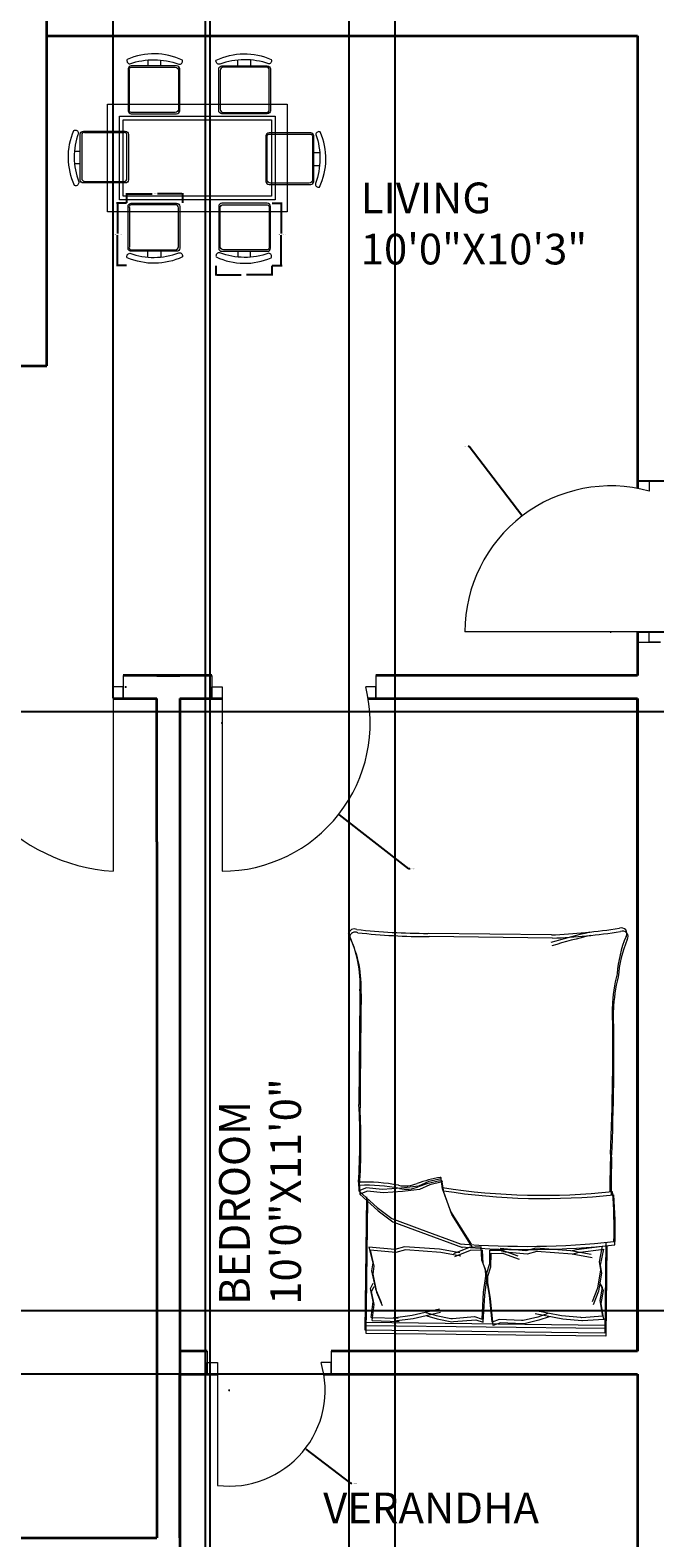
# Model space of a CAD drawing. Units: inches. Extents: x 1721 to 2510, y 1544 to 2360.
# Tile 3 of 10: x 1924 to 2046, y 1693 to 1988. Entities that reach past the tile are written whole.
import ezdxf

# ---------------------------------------------------------------- set-up
doc = ezdxf.new("R2010")
doc.units = ezdxf.units.IN
for name, color, linetype, lineweight in [('A-ANNO-DIMS', 2, 'Continuous', 18), ('A-AREA-IDEN', 7, 'Continuous', 18), ('A-DOOR', 3, 'Continuous', 18), ('A-FURN', 8, 'Continuous', 13), ('A-WALL', 7, 'Continuous', 35)]:
    doc.layers.add(name, color=color, linetype=linetype, lineweight=lineweight)
doc.styles.get("Standard").update_dxf_attribs({"font": 'arial.ttf'})
doc.dimstyles.get("Standard").update_dxf_attribs({"dimtxt": 0.18, "dimasz": 0.18, "dimexe": 0.18, "dimexo": 0.0625, "dimgap": 0.09, "dimtad": 0, "dimtih": 1, "dimtoh": 1, "dimdec": 4, "dimzin": 0, "dimdsep": 46, "dimtxsty": 'Standard', "dimcen": 0.09, "dimadec": 0, "dimazin": 0, "dimtfac": 1, "dimtdec": 4, "dimtofl": 0, "dimtmove": 0, "dimatfit": 3, "dimfxl": 1, "dimtolj": 1, "dimtzin": 0, "dimarcsym": 0})

# ---------------------------------------------------------------- blocks, each defined once
blk = doc.blocks.new('BED-DOUBLE')
for p, q in [((39.64, 78.43), (15.52, 78.72)), ((39.64, 78.43), (15.52, 78.72)), ((39.86, 77.8), (15.74, 78.09)), ((39.86, 77.8), (15.74, 78.09)), ((1.93, 30.11), (1.99, 28.4, 3.79)), ((1.93, 30.11), (1.99, 28.4, 3.79)), ((2.15, 29.48), (2.21, 27.77, 3.79)), ((2.15, 29.48), (2.21, 27.77, 3.79)), ((15.66, 30.21), (13.68, 29.32)), ((15.66, 30.21), (13.68, 29.32)), ((15.88, 29.58), (13.89, 28.69)), ((15.88, 29.58), (13.89, 28.69)), ((18.1, 30.79), (15.66, 30.21)), ((18.1, 30.79), (15.66, 30.21)), ((18.31, 30.16), (15.88, 29.58)), ((18.31, 30.16), (15.88, 29.58)), ((18.38, 28.81), (18.1, 30.79)), ((18.38, 28.81), (18.1, 30.79)), ((18.59, 28.18), (18.31, 30.16)), ((18.59, 28.18), (18.31, 30.16)), ((3.5, 28.99), (1.99, 28.4)), ((3.5, 28.99), (1.99, 28.4)), ((1.99, 28.4), (5.58, 25.17)), ((1.99, 28.4), (5.58, 25.17)), ((3.72, 28.36), (2.21, 27.77)), ((3.72, 28.36), (2.21, 27.77)), ((2.21, 27.77), (5.8, 24.54)), ((2.21, 27.77), (5.8, 24.54)), ((3.23, 1.19), (3.55, 27.27)), ((3.23, 1.19), (3.55, 27.27)), ((3.45, 0.56), (3.76, 26.64)), ((3.45, 0.56), (3.76, 26.64)), ((6.54, 28.65), (3.5, 28.99)), ((6.54, 28.65), (3.5, 28.99)), ((6.75, 28.02), (3.72, 28.36)), ((6.75, 28.02), (3.72, 28.36)), ((10.33, 28.91), (6.54, 28.65)), ((10.33, 28.91), (6.54, 28.65)), ((10.55, 28.28), (6.75, 28.02)), ((10.55, 28.28), (6.75, 28.02)), ((13.68, 29.32), (10.33, 28.91)), ((13.68, 29.32), (10.33, 28.91)), ((13.89, 28.69), (10.55, 28.28)), ((13.89, 28.69), (10.55, 28.28)), ((20, 24.39), (18.38, 28.81)), ((20, 24.39), (18.38, 28.81)), ((20.21, 23.76), (18.59, 28.18)), ((20.21, 23.76), (18.59, 28.18)), ((5.58, 25.17), (8.44, 23.01)), ((5.58, 25.17), (8.44, 23.01)), ((5.8, 24.54), (8.66, 22.38)), ((5.8, 24.54), (8.66, 22.38)), ((24.03, 17.98), (20, 24.39)), ((24.03, 17.98), (20, 24.39)), ((24.24, 17.35), (20.21, 23.76)), ((24.24, 17.35), (20.21, 23.76)), ((8.44, 23.01), (13.88, 20.98)), ((8.44, 23.01), (13.88, 20.98)), ((8.66, 22.38), (14.1, 20.35)), ((8.66, 22.38), (14.1, 20.35)), ((13.88, 20.98), (22.02, 18)), ((13.88, 20.98), (22.02, 18)), ((14.1, 20.35), (22.24, 17.37)), ((14.1, 20.35), (22.24, 17.37)), ((50.28, 18.38), (50.07, 0.63)), ((50.28, 18.38), (50.07, 0.63)), ((50.5, 17.75), (50.29, 0)), ((50.5, 17.75), (50.29, 0)), ((9.01, 16.97), (3.98, 17.42)), ((3.98, 17.42), (4.71, 14.34)), ((9.01, 16.97), (3.98, 17.42)), ((3.98, 17.42), (4.71, 14.34)), ((9.23, 16.34), (4.2, 16.8)), ((4.2, 16.8), (4.92, 13.71)), ((9.23, 16.34), (4.2, 16.8)), ((4.2, 16.8), (4.92, 13.71)), ((10.94, 17.49), (9.01, 16.97)), ((10.94, 17.49), (9.01, 16.97)), ((11.15, 16.86), (9.23, 16.34)), ((11.15, 16.86), (9.23, 16.34)), ((17.8, 16.99), (10.94, 17.49)), ((17.8, 16.99), (10.94, 17.49)), ((18.02, 16.36), (11.15, 16.86)), ((18.02, 16.36), (11.15, 16.86)), ((21.75, 16.29), (17.8, 16.99)), ((21.75, 16.29), (17.8, 16.99)), ((21.96, 15.66), (18.02, 16.36)), ((21.96, 15.66), (18.02, 16.36)), ((23.54, 17.35), (20.51, 16.13)), ((23.54, 17.35), (20.51, 16.13)), ((23.75, 16.73), (20.73, 15.5)), ((23.75, 16.73), (20.73, 15.5)), ((25.94, 17.48), (23.54, 17.35)), ((25.94, 17.48), (23.54, 17.35)), ((26.16, 16.85), (23.75, 16.73)), ((26.16, 16.85), (23.75, 16.73)), ((26.07, 14.85), (25.94, 17.48)), ((26.07, 14.85), (25.94, 17.48)), ((26.73, 13.04), (26.07, 14.85)), ((26.73, 13.04), (26.07, 14.85)), ((26.29, 14.22), (26.16, 16.85)), ((26.29, 14.22), (26.16, 16.85)), ((27.61, 14.21), (27.64, 16.84)), ((27.61, 14.21), (27.64, 16.84)), ((27.64, 16.84), (30.05, 16.81)), ((27.64, 16.84), (30.05, 16.81)), ((27.82, 13.58), (27.85, 16.21)), ((27.82, 13.58), (27.85, 16.21)), ((27.85, 16.21), (30.26, 16.18)), ((27.85, 16.21), (30.26, 16.18)), ((34.67, 16.66), (29.65, 17.12)), ((34.67, 16.66), (29.65, 17.12)), ((34.89, 16.03), (29.86, 16.49)), ((34.89, 16.03), (29.86, 16.49)), ((30.05, 16.81), (33.11, 15.7)), ((30.05, 16.81), (33.11, 15.7)), ((30.26, 16.18), (33.33, 15.07)), ((30.26, 16.18), (33.33, 15.07)), ((36.6, 17.19), (34.67, 16.66)), ((36.6, 17.19), (34.67, 16.66)), ((36.81, 16.56), (34.89, 16.03)), ((36.81, 16.56), (34.89, 16.03)), ((43.46, 16.68), (36.6, 17.19)), ((43.46, 16.68), (36.6, 17.19)), ((43.68, 16.05), (36.81, 16.56)), ((43.68, 16.05), (36.81, 16.56)), ((43.46, 16.68), (44.58, 16.98)), ((43.46, 16.68), (44.58, 16.98)), ((47.41, 15.98), (43.46, 16.68)), ((47.41, 15.98), (43.46, 16.68)), ((43.68, 16.05), (44.79, 16.35)), ((43.68, 16.05), (44.79, 16.35)), ((47.62, 15.35), (43.68, 16.05)), ((47.62, 15.35), (43.68, 16.05)), ((44.58, 16.98), (49.58, 17.63)), ((44.58, 16.98), (49.58, 17.63)), ((44.79, 16.35), (49.8, 17)), ((44.79, 16.35), (49.8, 17)), ((49.58, 17.63), (48.98, 14.52)), ((49.58, 17.63), (48.98, 14.52)), ((49.8, 17), (49.19, 13.89)), ((49.8, 17), (49.19, 13.89)), ((4.71, 14.34), (4.5, 12.77)), ((4.71, 14.34), (4.5, 12.77)), ((4.5, 12.77), (5.25, 9.26)), ((4.5, 12.77), (5.25, 9.26)), ((4.92, 13.71), (4.72, 12.14)), ((4.92, 13.71), (4.72, 12.14)), ((4.72, 12.14), (5.46, 8.63)), ((4.72, 12.14), (5.46, 8.63)), ((26.95, 12.41), (26.29, 14.22)), ((26.95, 12.41), (26.29, 14.22)), ((26.8, 11.77), (26.73, 13.04)), ((26.8, 11.77), (26.73, 13.04)), ((27.01, 11.14), (26.95, 12.41)), ((27.01, 11.14), (26.95, 12.41)), ((27, 11.1), (27.02, 12.38)), ((27, 11.1), (27.02, 12.38)), ((27.02, 12.38), (27.61, 14.21)), ((27.02, 12.38), (27.61, 14.21)), ((27.23, 11.75), (27.82, 13.58)), ((27.23, 11.75), (27.82, 13.58)), ((49.24, 12.96), (48.63, 9.42)), ((49.24, 12.96), (48.63, 9.42)), ((49.46, 12.33), (48.85, 8.79)), ((49.46, 12.33), (48.85, 8.79)), ((48.98, 14.52), (49.24, 12.96)), ((48.98, 14.52), (49.24, 12.96)), ((49.19, 13.89), (49.46, 12.33)), ((49.19, 13.89), (49.46, 12.33)), ((4.25, 9.35), (4.77, 10.37)), ((4.25, 9.35), (4.77, 10.37)), ((4.8, 6.82), (4.25, 9.35)), ((4.8, 6.82), (4.25, 9.35)), ((4.47, 8.72), (4.98, 9.74)), ((4.47, 8.72), (4.98, 9.74)), ((5.25, 9.26), (6.37, 6.62)), ((5.25, 9.26), (6.37, 6.62)), ((26.39, 8.62), (26.8, 11.77)), ((26.39, 8.62), (26.8, 11.77)), ((26.61, 7.99), (27.01, 11.14)), ((26.61, 7.99), (27.01, 11.14)), ((27.53, 7.98), (27, 11.1)), ((27.53, 7.98), (27, 11.1)), ((27.22, 10.47), (27.23, 11.75)), ((27.22, 10.47), (27.23, 11.75)), ((27.75, 7.35), (27.22, 10.47)), ((27.75, 7.35), (27.22, 10.47)), ((48.63, 9.42), (47.61, 6.74)), ((48.63, 9.42), (47.61, 6.74)), ((49.63, 9.55), (49.07, 10.55)), ((49.63, 9.55), (49.07, 10.55)), ((49.17, 7.01), (49.63, 9.55)), ((49.17, 7.01), (49.63, 9.55)), ((49.84, 8.92), (49.29, 9.92)), ((49.84, 8.92), (49.29, 9.92)), ((49.39, 6.38), (49.84, 8.92)), ((49.39, 6.38), (49.84, 8.92)), ((4.39, 3.68), (4.8, 6.82)), ((4.39, 3.68), (4.8, 6.82)), ((5.02, 6.19), (4.47, 8.72)), ((5.02, 6.19), (4.47, 8.72)), ((4.61, 3.05), (5.02, 6.19)), ((4.61, 3.05), (5.02, 6.19)), ((5.46, 8.63), (6.59, 5.99)), ((5.46, 8.63), (6.59, 5.99)), ((26.09, 3.36), (26.39, 8.62)), ((26.09, 3.36), (26.39, 8.62)), ((26.3, 2.73), (26.61, 7.99)), ((26.3, 2.73), (26.61, 7.99)), ((28.04, 2.73), (27.53, 7.98)), ((28.04, 2.73), (27.53, 7.98)), ((28.25, 2.1), (27.75, 7.35)), ((28.25, 2.1), (27.75, 7.35)), ((48.85, 8.79), (47.82, 6.11)), ((48.85, 8.79), (47.82, 6.11)), ((49.7, 3.88), (49.17, 7.01)), ((49.7, 3.88), (49.17, 7.01)), ((49.92, 3.25), (49.39, 6.38)), ((49.92, 3.25), (49.39, 6.38)), ((4.39, 3.68), (9.69, 3.52)), ((4.39, 3.68), (9.69, 3.52)), ((4.61, 3.05), (9.9, 2.89)), ((4.61, 3.05), (9.9, 2.89)), ((8.71, 3.62), (12.44, 4.09)), ((8.71, 3.62), (12.44, 4.09)), ((9.69, 3.52), (8.71, 3.62)), ((9.69, 3.52), (8.71, 3.62)), ((8.92, 2.99), (12.65, 3.46)), ((8.92, 2.99), (12.65, 3.46)), ((9.9, 2.89), (8.92, 2.99)), ((9.9, 2.89), (8.92, 2.99)), ((12.44, 4.09), (17.76, 5.35)), ((12.44, 4.09), (17.76, 5.35)), ((12.65, 3.46), (17.98, 4.72)), ((12.65, 3.46), (17.98, 4.72)), ((15.1, 4.65), (17.12, 4.04)), ((15.1, 4.65), (17.12, 4.04)), ((15.32, 4.02), (17.34, 3.41)), ((15.32, 4.02), (17.34, 3.41)), ((17.12, 4.04), (19.98, 3.48)), ((17.12, 4.04), (19.98, 3.48)), ((17.34, 3.41), (20.2, 2.85)), ((17.34, 3.41), (20.2, 2.85)), ((19.98, 3.48), (20.3, 3.49)), ((19.98, 3.48), (20.3, 3.49)), ((20.3, 3.49), (24.64, 3.85)), ((20.3, 3.49), (24.64, 3.85)), ((20.52, 2.86), (24.86, 3.22)), ((20.52, 2.86), (24.86, 3.22)), ((24.64, 3.85), (26.09, 3.36)), ((24.64, 3.85), (26.09, 3.36)), ((24.86, 3.22), (26.3, 2.73)), ((24.86, 3.22), (26.3, 2.73)), ((29.46, 3.28), (28.04, 2.73)), ((29.46, 3.28), (28.04, 2.73)), ((33.81, 3.08), (29.46, 3.28)), ((33.81, 3.08), (29.46, 3.28)), ((34.13, 3.08), (33.81, 3.08)), ((34.13, 3.08), (33.81, 3.08)), ((36.97, 3.75), (34.13, 3.08)), ((36.97, 3.75), (34.13, 3.08)), ((37.19, 3.12), (34.35, 2.45)), ((37.19, 3.12), (34.35, 2.45)), ((41.65, 3.98), (36.28, 5.04)), ((41.65, 3.98), (36.28, 5.04)), ((41.87, 3.35), (36.49, 4.41)), ((41.87, 3.35), (36.49, 4.41)), ((38.96, 4.44), (36.97, 3.75)), ((38.96, 4.44), (36.97, 3.75)), ((39.18, 3.81), (37.19, 3.12)), ((39.18, 3.81), (37.19, 3.12)), ((45.39, 3.65), (41.65, 3.98)), ((45.39, 3.65), (41.65, 3.98)), ((45.61, 3.02), (41.87, 3.35)), ((45.61, 3.02), (41.87, 3.35)), ((45.5, 3.63), (45.39, 3.65)), ((45.5, 3.63), (45.39, 3.65)), ((49.7, 3.91), (45.5, 3.63)), ((49.7, 3.91), (45.5, 3.63)), ((45.71, 3), (45.61, 3.02)), ((45.71, 3), (45.61, 3.02)), ((49.91, 3.28), (45.71, 3)), ((49.91, 3.28), (45.71, 3)), ((50.07, 0.63), (3.23, 1.19)), ((50.07, 0.63), (3.23, 1.19)), ((50.09, 2.13), (3.25, 2.69)), ((50.09, 2.13), (3.25, 2.69)), ((50.29, 0), (3.45, 0.56)), ((50.29, 0), (3.45, 0.56)), ((50.31, 1.5), (3.47, 2.06)), ((50.31, 1.5), (3.47, 2.06)), ((20.2, 2.85), (20.52, 2.86)), ((20.2, 2.85), (20.52, 2.86)), ((29.68, 2.65), (28.25, 2.1)), ((29.68, 2.65), (28.25, 2.1)), ((34.03, 2.45), (29.68, 2.65)), ((34.03, 2.45), (29.68, 2.65)), ((34.35, 2.45), (34.03, 2.45)), ((34.35, 2.45), (34.03, 2.45))]:
    blk.add_line(p, q)
for centre, radius, start, end in [((1.08, 78.52), 1.08, 61.9736, 175.3348), ((1.08, 78.52), 1.08, 61.9736, 175.3348), ((34.83, 197.67), 119.34, 272.3106, 278.7239), ((34.83, 197.67), 119.34, 272.3106, 278.7239), ((53.35, 78.73), 1.07, 325.4884, 112.793), ((53.35, 78.73), 1.07, 325.4884, 112.793), ((-20.36, 68.78), 22.61, 356.7862, 25.7829), ((-20.36, 68.78), 22.61, 356.7862, 25.7829), ((1.29, 77.89), 1.08, 61.9736, 175.3348), ((1.29, 77.89), 1.08, 61.9736, 175.3348), ((-20.14, 68.15), 22.61, 356.7862, 25.7829), ((-20.14, 68.15), 22.61, 356.7862, 25.7829), ((15.63, 209.12), 130.4, 263.8146, 269.9499), ((15.63, 209.12), 130.4, 263.8146, 269.9499), ((15.85, 208.49), 130.4, 263.8146, 269.9499), ((15.85, 208.49), 130.4, 263.8146, 269.9499), ((70.08, -22.85), 104.34, 102.698, 107.0202), ((70.08, -22.85), 104.34, 102.698, 107.0202), ((70.29, -23.48), 104.34, 102.698, 107.0202), ((70.29, -23.48), 104.34, 102.698, 107.0202), ((35.05, 197.04), 119.34, 272.3106, 278.7239), ((35.05, 197.04), 119.34, 272.3106, 278.7239), ((75.53, 69.21), 23.09, 157.2899, 175.9668), ((75.53, 69.21), 23.09, 157.2899, 175.9668), ((75.75, 68.58), 23.09, 157.2899, 175.9668), ((75.75, 68.58), 23.09, 157.2899, 175.9668), ((53.56, 78.1), 1.07, 325.4884, 112.793), ((53.56, 78.1), 1.07, 325.4884, 112.793), ((80.6, 63.5), 29.05, 165.3797, 178.2261), ((80.6, 63.5), 29.05, 165.3797, 178.2261), ((80.81, 62.87), 29.05, 165.3797, 178.2261), ((80.81, 62.87), 29.05, 165.3797, 178.2261), ((4473.12, 14.21), 4471.22, 179.317, 179.60172), ((4473.12, 14.21), 4471.22, 179.317, 179.60172), ((4473.34, 13.58), 4471.22, 179.317, 179.60172), ((4473.34, 13.58), 4471.22, 179.317, 179.60172), ((-421.08, 55.88), 472.73, 357.5425, 1.0334), ((-421.08, 55.88), 472.73, 357.5425, 1.0334), ((-420.87, 55.25), 472.73, 357.5425, 1.0334), ((-420.87, 55.25), 472.73, 357.5425, 1.0334), ((-124.73, 38.32), 126.93, 356.294, 3.1513), ((-124.73, 38.32), 126.93, 356.294, 3.1513), ((-124.51, 37.69), 126.93, 356.294, 3.1513), ((-124.51, 37.69), 126.93, 356.294, 3.1513), ((217.81, 29.18), 166.73, 177.791, 180.323), ((217.81, 29.18), 166.73, 177.791, 180.323), ((218.03, 28.55), 166.73, 177.791, 180.323), ((218.03, 28.55), 166.73, 177.791, 180.323), ((3.1, -5.33), 35.46, 79.1911, 91.8805), ((3.1, -5.33), 35.46, 79.1911, 91.8805), ((3.31, -5.96), 35.46, 79.1911, 91.8805), ((3.31, -5.96), 35.46, 79.1911, 91.8805), ((11.02, 35.47), 6.1, 257.9756, 293.0532), ((11.02, 35.47), 6.1, 257.9756, 293.0532), ((22.96, 2.41), 29.06, 99.9765, 109.1954), ((22.96, 2.41), 29.06, 99.9765, 109.1954), ((23.18, 1.78), 29.06, 99.9765, 109.1954), ((23.18, 1.78), 29.06, 99.9765, 109.1954), ((17.93, 30.85), 0.181, 339.5612, 90.4525), ((17.93, 30.85), 0.181, 339.5612, 90.4525), ((18.15, 30.22), 0.181, 339.5612, 90.4525), ((18.15, 30.22), 0.181, 339.5612, 90.4525), ((11.23, 34.84), 6.1, 257.9756, 293.0532), ((11.23, 34.84), 6.1, 257.9756, 293.0532), ((37.91, 154), 126.46, 261.0993, 276.2154), ((37.91, 154), 126.46, 261.0993, 276.2154), ((38.12, 153.37), 126.46, 261.0993, 276.2154), ((38.12, 153.37), 126.46, 261.0993, 276.2154), ((-29.75, 21.28), 81.65, 358.0366, 4.9188), ((-29.75, 21.28), 81.65, 358.0366, 4.9188), ((-29.53, 20.65), 81.65, 358.0366, 4.9188), ((-29.53, 20.65), 81.65, 358.0366, 4.9188), ((34.68, 179.26), 161.69, 265.4014, 276.097), ((34.68, 179.26), 161.69, 265.4014, 276.097), ((34.89, 178.63), 161.69, 265.4014, 276.097), ((34.89, 178.63), 161.69, 265.4014, 276.097)]:
    blk.add_arc(centre, radius, start, end)
blk = doc.blocks.new('TABLE-DINING-RECT')
for points in [[(0, 21.04), (35.07, 21.04), (35.07, 0), (0, 0)], [(2.34, 18.71), (32.73, 18.71), (32.73, 2.34), (2.34, 2.34)], [(3.04, 18), (32.03, 18), (32.03, 3.04), (3.04, 3.04)]]:
    blk.add_lwpolyline(points, close=True)
blk = doc.blocks.new('CHAIR-DINING-B')
for points in [[(9.72, 2.34), (0.85, 2.34, -0.414214), (0.23, 2.96), (0.23, 11.11, -0.414214), (0.85, 11.73), (9.72, 11.73, -0.414214), (10.34, 11.11), (10.34, 2.96, -0.414214), (9.72, 2.34)], [(10.13, 2.03, -0.578392), (10.85, 1.23, -0.214524), (0.07, 1.08, -0.552014), (0.57, 1.95, 0.175809), (10.13, 2.03)], [(6.61, 2.34), (6.61, 1.21, 0.064759)]]:
    blk.add_lwpolyline(points, format="xyb")
blk.add_lwpolyline([(0.86, 2.62), (9.44, 2.62, 0.414214), (10.06, 3.24), (10.06, 10.83, 0.414214), (9.44, 11.45), (0.86, 11.45, 0.512069), (0.51, 10.83), (0.51, 3.24, 0.512069)], format="xyb", close=True)
blk.add_lwpolyline([(4.12, 1.19), (4.12, 2.34)])
blk = doc.blocks.new('CHAIR-DINING-C')
for points in [[(10.03, 2.34, 0.414214), (10.65, 2.96), (10.65, 11.11, 0.414214), (10.03, 11.73), (1.16, 11.73, 0.414214), (0.54, 11.11), (0.54, 2.96, 0.414214), (1.16, 2.34), (10.03, 2.34)], [(10.31, 1.95, -0.175809), (0.75, 2.03, 0.578392), (0.03, 1.23, 0.214524), (10.81, 1.08, 0.552014), (10.31, 1.95, -0.065079)], [(4.27, 2.34), (4.27, 1.21, -0.064759)]]:
    blk.add_lwpolyline(points, format="xyb")
blk.add_lwpolyline([(10.02, 2.62), (1.44, 2.62, -0.414214), (0.82, 3.24), (0.82, 10.83, -0.414214), (1.44, 11.45), (10.02, 11.45, -0.512069), (10.37, 10.83), (10.37, 3.24, -0.512069)], format="xyb", close=True)
blk.add_lwpolyline([(6.76, 1.19), (6.76, 2.34)])
blk = doc.blocks.new('*D32')
at = {"layer": 'A-ANNO-DIMS', "color": 0, "lineweight": -2, "transparency": 16777216}
for p, q in [((1942.57, 1953.89), (1940.63, 1953.89)), ((1940.81, 1953.71), (1940.81, 1948.01)), ((1940.81, 1941.93), (1940.81, 1947.64)), ((1942.57, 1941.75), (1940.63, 1941.75))]:
    blk.add_line(p, q, dxfattribs=at)
at = {"layer": 'A-ANNO-DIMS', "color": 0, "transparency": 16777216}
for points in [[(1940.78, 1953.71), (1940.84, 1953.71), (1940.81, 1953.89)], [(1940.78, 1941.93), (1940.84, 1941.93), (1940.81, 1941.75)]]:
    blk.add_solid(points, dxfattribs=at)
at = {"layer": 'Defpoints', "color": 0, "transparency": 16777216}
for p in [(1940.81, 1953.89), (1942.63, 1953.89), (1942.63, 1941.75)]:
    blk.add_point(p, dxfattribs=at)
at = {"layer": 'A-ANNO-DIMS', "color": 0, "transparency": 16777216, "insert": (1940.81, 1947.82), "char_height": 0.18, "attachment_point": 5}
blk.add_mtext('\\A1;CHAIR B 12 TYP.', dxfattribs=at)
blk = doc.blocks.new('*D33')
at = {"layer": 'A-ANNO-DIMS', "color": 0, "lineweight": -2, "transparency": 16777216}
for p, q in [((1942.63, 1953.96), (1942.63, 1955.89)), ((1942.81, 1955.71), (1947.58, 1955.71)), ((1953.4, 1955.71), (1948.62, 1955.71)), ((1953.58, 1953.96), (1953.58, 1955.89))]:
    blk.add_line(p, q, dxfattribs=at)
at = {"layer": 'A-ANNO-DIMS', "color": 0, "transparency": 16777216}
for points in [[(1942.81, 1955.74), (1942.81, 1955.68), (1942.63, 1955.71)], [(1953.4, 1955.74), (1953.4, 1955.68), (1953.58, 1955.71)]]:
    blk.add_solid(points, dxfattribs=at)
at = {"layer": 'Defpoints', "color": 0, "transparency": 16777216}
for p in [(1942.63, 1953.89), (1953.58, 1955.71), (1953.58, 1953.89)]:
    blk.add_point(p, dxfattribs=at)
at = {"layer": 'A-ANNO-DIMS', "color": 0, "transparency": 16777216, "insert": (1948.1, 1955.71), "char_height": 0.18, "attachment_point": 5}
blk.add_mtext('\\A1;11 TYP.', dxfattribs=at)
blk = doc.blocks.new('*D34')
at = {"layer": 'A-ANNO-DIMS', "color": 0, "lineweight": -2, "transparency": 16777216}
for p, q in [((1971.04, 1953.89), (1972.98, 1953.89)), ((1972.8, 1953.71), (1972.8, 1948.01)), ((1972.8, 1941.93), (1972.8, 1947.64)), ((1971.04, 1941.75), (1972.98, 1941.75))]:
    blk.add_line(p, q, dxfattribs=at)
at = {"layer": 'A-ANNO-DIMS', "color": 0, "transparency": 16777216}
for points in [[(1972.77, 1953.71), (1972.83, 1953.71), (1972.8, 1953.89)], [(1972.77, 1941.93), (1972.83, 1941.93), (1972.8, 1941.75)]]:
    blk.add_solid(points, dxfattribs=at)
at = {"layer": 'Defpoints', "color": 0, "transparency": 16777216}
for p in [(1970.98, 1953.89), (1972.8, 1953.89), (1970.98, 1941.75)]:
    blk.add_point(p, dxfattribs=at)
at = {"layer": 'A-ANNO-DIMS', "color": 0, "transparency": 16777216, "insert": (1972.8, 1947.82), "char_height": 0.18, "attachment_point": 5}
blk.add_mtext('\\A1;CHAIR C 12 TYP.', dxfattribs=at)
blk = doc.blocks.new('*D35')
at = {"layer": 'A-ANNO-DIMS', "color": 0, "lineweight": -2, "transparency": 16777216}
for p, q in [((1960.04, 1941.69), (1960.04, 1939.75)), ((1970.98, 1941.69), (1970.98, 1939.75)), ((1960.22, 1939.93), (1964.99, 1939.93)), ((1970.8, 1939.93), (1966.03, 1939.93))]:
    blk.add_line(p, q, dxfattribs=at)
at = {"layer": 'A-ANNO-DIMS', "color": 0, "transparency": 16777216}
for points in [[(1960.22, 1939.96), (1960.22, 1939.9), (1960.04, 1939.93)], [(1970.8, 1939.96), (1970.8, 1939.9), (1970.98, 1939.93)]]:
    blk.add_solid(points, dxfattribs=at)
at = {"layer": 'Defpoints', "color": 0, "transparency": 16777216}
for p in [(1960.04, 1941.75), (1970.98, 1941.75), (1970.98, 1939.93)]:
    blk.add_point(p, dxfattribs=at)
at = {"layer": 'A-ANNO-DIMS', "color": 0, "transparency": 16777216, "insert": (1965.51, 1939.93), "char_height": 0.18, "attachment_point": 5}
blk.add_mtext('\\A1;11 TYP.', dxfattribs=at)
blk = doc.blocks.new('*D53')
at = {"layer": 'A-ANNO-DIMS', "color": 0, "lineweight": -2, "transparency": 16777216}
for p, q in [((2127.44, 1854.49), (1765.42, 1854.49)), ((1765.6, 1854.31), (1765.6, 1796.17)), ((1765.6, 1737.67), (1765.6, 1795.81)), ((2127.44, 1737.49), (1765.42, 1737.49))]:
    blk.add_line(p, q, dxfattribs=at)
at = {"layer": 'A-ANNO-DIMS', "color": 0, "transparency": 16777216}
for points in [[(1765.57, 1854.31), (1765.63, 1854.31), (1765.6, 1854.49)], [(1765.57, 1737.67), (1765.63, 1737.67), (1765.6, 1737.49)]]:
    blk.add_solid(points, dxfattribs=at)
at = {"layer": 'Defpoints', "color": 0, "transparency": 16777216}
for p in [(1765.6, 1854.49), (2127.5, 1854.49), (2127.5, 1737.49)]:
    blk.add_point(p, dxfattribs=at)
at = {"layer": 'A-ANNO-DIMS', "color": 0, "transparency": 16777216, "insert": (1765.6, 1795.99), "char_height": 0.18, "attachment_point": 5}
blk.add_mtext('\\A1;117', dxfattribs=at)
blk = doc.blocks.new('*D58')
at = {"layer": 'A-ANNO-DIMS', "color": 0, "lineweight": -2, "transparency": 16777216}
for p, q in [((2042.56, 1899.66), (2409.08, 1899.66)), ((2408.9, 1899.48), (2408.9, 1885.09)), ((2408.9, 1870.34), (2408.9, 1884.73)), ((2042.56, 1870.16), (2409.08, 1870.16))]:
    blk.add_line(p, q, dxfattribs=at)
at = {"layer": 'A-ANNO-DIMS', "color": 0, "transparency": 16777216}
for points in [[(2408.87, 1899.48), (2408.93, 1899.48), (2408.9, 1899.66)], [(2408.87, 1870.34), (2408.93, 1870.34), (2408.9, 1870.16)]]:
    blk.add_solid(points, dxfattribs=at)
at = {"layer": 'Defpoints', "color": 0, "transparency": 16777216}
for p in [(2042.5, 1899.66), (2408.9, 1899.66), (2042.5, 1870.16)]:
    blk.add_point(p, dxfattribs=at)
at = {"layer": 'A-ANNO-DIMS', "color": 0, "transparency": 16777216, "insert": (2408.9, 1884.91), "char_height": 0.18, "attachment_point": 5}
blk.add_mtext('\\A1;29.505', dxfattribs=at)
blk = doc.blocks.new('*D59')
at = {"layer": 'A-ANNO-DIMS', "color": 0, "lineweight": -2, "transparency": 16777216}
for p, q in [((1904.34, 1857.19), (1904.34, 2317.71)), ((1904.52, 2317.53), (1921.76, 2317.53)), ((1939.78, 2317.53), (1922.54, 2317.53)), ((1939.96, 1857.19), (1939.96, 2317.71))]:
    blk.add_line(p, q, dxfattribs=at)
at = {"layer": 'A-ANNO-DIMS', "color": 0, "transparency": 16777216}
for points in [[(1904.52, 2317.56), (1904.52, 2317.5), (1904.34, 2317.53)], [(1939.78, 2317.56), (1939.78, 2317.5), (1939.96, 2317.53)]]:
    blk.add_solid(points, dxfattribs=at)
at = {"layer": 'Defpoints', "color": 0, "transparency": 16777216}
for p in [(1939.96, 2317.53), (1904.34, 1857.13), (1939.96, 1857.13)]:
    blk.add_point(p, dxfattribs=at)
at = {"layer": 'A-ANNO-DIMS', "color": 0, "transparency": 16777216, "insert": (1922.15, 2317.53), "char_height": 0.18, "attachment_point": 5}
blk.add_mtext('\\A1;35.62', dxfattribs=at)
blk = doc.blocks.new('*D62')
at = {"layer": 'A-ANNO-DIMS', "color": 0, "lineweight": -2, "transparency": 16777216}
for p, q in [((1957.99, 2252.88), (1957.99, 1606.75)), ((1986.02, 2252.88), (1986.02, 1606.75)), ((1958.17, 1606.93), (1971.61, 1606.93)), ((1985.84, 1606.93), (1972.4, 1606.93))]:
    blk.add_line(p, q, dxfattribs=at)
at = {"layer": 'A-ANNO-DIMS', "color": 0, "transparency": 16777216}
for points in [[(1958.17, 1606.96), (1958.17, 1606.9), (1957.99, 1606.93)], [(1985.84, 1606.96), (1985.84, 1606.9), (1986.02, 1606.93)]]:
    blk.add_solid(points, dxfattribs=at)
at = {"layer": 'Defpoints', "color": 0, "transparency": 16777216}
for p in [(1957.99, 2252.94), (1986.02, 2252.94), (1986.02, 1606.93)]:
    blk.add_point(p, dxfattribs=at)
at = {"layer": 'A-ANNO-DIMS', "color": 0, "transparency": 16777216, "insert": (1972.01, 1606.93), "char_height": 0.18, "attachment_point": 5}
blk.add_mtext('\\A1;28.03', dxfattribs=at)
blk = doc.blocks.new('*D63')
at = {"layer": 'A-ANNO-DIMS', "color": 0, "lineweight": -2, "transparency": 16777216}
for p, q in [((1958.89, 2116.38), (1958.89, 1606.75)), ((1995.05, 2116.38), (1995.05, 1606.75)), ((1959.07, 1606.93), (1976.58, 1606.93)), ((1994.87, 1606.93), (1977.36, 1606.93))]:
    blk.add_line(p, q, dxfattribs=at)
at = {"layer": 'A-ANNO-DIMS', "color": 0, "transparency": 16777216}
for points in [[(1959.07, 1606.96), (1959.07, 1606.9), (1958.89, 1606.93)], [(1994.87, 1606.96), (1994.87, 1606.9), (1995.05, 1606.93)]]:
    blk.add_solid(points, dxfattribs=at)
at = {"layer": 'Defpoints', "color": 0, "transparency": 16777216}
for p in [(1958.89, 2116.44), (1995.05, 2116.44), (1995.05, 1606.93)]:
    blk.add_point(p, dxfattribs=at)
at = {"layer": 'A-ANNO-DIMS', "color": 0, "transparency": 16777216, "insert": (1976.97, 1606.93), "char_height": 0.18, "attachment_point": 5}
blk.add_mtext('\\A1;36.16', dxfattribs=at)
blk = doc.blocks.new('*D67')
at = {"layer": 'A-ANNO-DIMS', "color": 0, "lineweight": -2, "transparency": 16777216}
for p, q in [((2042.44, 1725.13), (1765.42, 1725.13)), ((1765.6, 1724.95), (1765.6, 1707.06)), ((1765.6, 1688.81), (1765.6, 1706.7)), ((2042.44, 1688.63), (1765.42, 1688.63))]:
    blk.add_line(p, q, dxfattribs=at)
at = {"layer": 'A-ANNO-DIMS', "color": 0, "transparency": 16777216}
for points in [[(1765.57, 1724.95), (1765.63, 1724.95), (1765.6, 1725.13)], [(1765.57, 1688.81), (1765.63, 1688.81), (1765.6, 1688.63)]]:
    blk.add_solid(points, dxfattribs=at)
at = {"layer": 'Defpoints', "color": 0, "transparency": 16777216}
for p in [(1765.6, 1725.13), (2042.5, 1725.13), (2042.5, 1688.63)]:
    blk.add_point(p, dxfattribs=at)
at = {"layer": 'A-ANNO-DIMS', "color": 0, "transparency": 16777216, "insert": (1765.6, 1706.88), "char_height": 0.18, "attachment_point": 5}
blk.add_mtext('\\A1;36.5', dxfattribs=at)
blk = doc.blocks.new('*D73')
at = {"layer": 'A-ANNO-DIMS', "color": 0, "lineweight": -2, "transparency": 16777216}
for p, q in [((1942.33, 1859.38), (1942.51, 1859.38)), ((1942.42, 1859.29), (1942.42, 1859.47)), ((1900.23, 1819.97), (1915.92, 1834.63)), ((1900.05, 1819.97), (1900.23, 1819.97))]:
    blk.add_line(p, q, dxfattribs=at)
at = {"layer": 'A-ANNO-DIMS', "color": 0, "transparency": 16777216}
blk.add_solid([(1915.9, 1834.65), (1915.94, 1834.61), (1916.05, 1834.75)], dxfattribs=at)
at = {"layer": 'Defpoints', "color": 0, "transparency": 16777216}
for p in [(1942.42, 1859.38), (1916.05, 1834.75)]:
    blk.add_point(p, dxfattribs=at)
at = {"layer": 'A-ANNO-DIMS', "color": 0, "transparency": 16777216, "insert": (1899.5, 1819.97), "char_height": 0.18, "attachment_point": 5}
blk.add_mtext('\\A1;R36.084', dxfattribs=at)
blk = doc.blocks.new('*D79')
at = {"layer": 'A-ANNO-DIMS', "color": 0, "lineweight": -2, "transparency": 16777216}
for p, q in [((1961.16, 1852.35), (1961.34, 1852.35)), ((1961.25, 1852.26), (1961.25, 1852.44)), ((1997.79, 1823.83), (1984.23, 1834.41)), ((1997.97, 1823.83), (1997.79, 1823.83))]:
    blk.add_line(p, q, dxfattribs=at)
at = {"layer": 'A-ANNO-DIMS', "color": 0, "transparency": 16777216}
blk.add_solid([(1984.25, 1834.44), (1984.21, 1834.39), (1984.09, 1834.52)], dxfattribs=at)
at = {"layer": 'Defpoints', "color": 0, "transparency": 16777216}
for p in [(1961.25, 1852.35), (1984.09, 1834.52)]:
    blk.add_point(p, dxfattribs=at)
at = {"layer": 'A-ANNO-DIMS', "color": 0, "transparency": 16777216, "insert": (1998.45, 1823.83), "char_height": 0.18, "attachment_point": 5}
blk.add_mtext('\\A1;R28.97', dxfattribs=at)
blk = doc.blocks.new('*D80')
at = {"layer": 'A-ANNO-DIMS', "color": 0, "lineweight": -2, "transparency": 16777216}
for p, q in [((2009.39, 1906.4), (2009.57, 1906.4)), ((2009.57, 1906.4), (2019.84, 1892.96)), ((2037.17, 1870.16), (2037.35, 1870.16)), ((2037.26, 1870.07), (2037.26, 1870.25))]:
    blk.add_line(p, q, dxfattribs=at)
at = {"layer": 'A-ANNO-DIMS', "color": 0, "transparency": 16777216}
blk.add_solid([(2019.87, 1892.97), (2019.82, 1892.94), (2019.95, 1892.81)], dxfattribs=at)
at = {"layer": 'Defpoints', "color": 0, "transparency": 16777216}
for p in [(2019.95, 1892.81), (2037.26, 1870.16)]:
    blk.add_point(p, dxfattribs=at)
at = {"layer": 'A-ANNO-DIMS', "color": 0, "transparency": 16777216, "insert": (2008.93, 1906.4), "char_height": 0.18, "attachment_point": 5}
blk.add_mtext('\\A1;R28.51', dxfattribs=at)
blk = doc.blocks.new('*D94')
at = {"layer": 'A-ANNO-DIMS', "color": 0, "lineweight": -2, "transparency": 16777216}
for p, q in [((1962.58, 1721.98), (1962.76, 1721.98)), ((1962.67, 1721.89), (1962.67, 1722.07)), ((1986.47, 1703.74), (1977.69, 1710.47)), ((1986.65, 1703.74), (1986.47, 1703.74))]:
    blk.add_line(p, q, dxfattribs=at)
at = {"layer": 'A-ANNO-DIMS', "color": 0, "transparency": 16777216}
blk.add_solid([(1977.71, 1710.5), (1977.67, 1710.45), (1977.55, 1710.58)], dxfattribs=at)
at = {"layer": 'Defpoints', "color": 0, "transparency": 16777216}
for p in [(1962.67, 1721.98), (1977.55, 1710.58)]:
    blk.add_point(p, dxfattribs=at)
at = {"layer": 'A-ANNO-DIMS', "color": 0, "transparency": 16777216, "insert": (1987.13, 1703.74), "char_height": 0.18, "attachment_point": 5}
blk.add_mtext('\\A1;R18.74', dxfattribs=at)

msp = doc.modelspace()

# ---------------------------------------------------------------- linework, layer by layer
at = {"layer": 'A-DOOR'}
for p, q in [((2042.5024, 1899.6648), (2047.0024, 1899.6648)), ((2047.0024, 1899.6648), (2044.7524, 1899.6648)), ((2044.7524, 1899.6648), (2044.7524, 1897.6648)), ((2044.7524, 1870.1595), (2008.7524, 1870.1595)), ((2042.5024, 1868.1595), (2047.0024, 1868.1595)), ((2044.7524, 1868.1595), (2044.7524, 1870.1595)), ((2047.0024, 1868.1595), (2044.7524, 1868.1595)), ((1941.9594, 1859.3798), (1939.9594, 1859.3798)), ((1939.9594, 1859.3798), (1939.9594, 1823.3798)), ((1941.9594, 1861.6298), (1941.9594, 1857.1298)), ((1941.9594, 1857.1298), (1941.9594, 1859.3798)), ((1959.2534, 1861.6298), (1959.2534, 1857.1298)), ((1959.2534, 1857.1298), (1959.2534, 1859.3798)), ((1959.2534, 1859.3798), (1959.2534, 1859.3798)), ((1959.2534, 1859.3798), (1961.2534, 1859.3798)), ((1961.2534, 1859.3798), (1961.2534, 1823.3798)), ((1991.3565, 1859.3798), (1989.3565, 1859.3798)), ((1991.3565, 1861.6298), (1991.3565, 1857.1298)), ((1991.3565, 1857.1298), (1991.3565, 1859.3798)), ((1958.3569, 1729.6298), (1958.3569, 1725.1298)), ((1982.6146, 1729.6298), (1982.6146, 1725.1298)), ((1958.3569, 1725.1298), (1958.3569, 1727.3798)), ((1958.3569, 1727.3798), (1960.3569, 1727.3798)), ((1960.3569, 1727.3798), (1960.3569, 1703.3798)), ((1982.6146, 1727.3798), (1980.6146, 1727.3798)), ((1982.6146, 1725.1298), (1982.6146, 1727.3798))]:
    msp.add_line(p, q, dxfattribs=at)
for centre, radius, start, end in [((2037.2599, 1870.1595), 28.5075, 74.762217, 180), ((1942.4229, 1859.3798), 36.0842, 180, 266.085268), ((1961.2534, 1852.349), 28.9692, 270, 14.045862), ((1962.6688, 1721.9779), 18.7412, 262.914002, 16.75258)]:
    msp.add_arc(centre, radius, start, end, dxfattribs=at)
at = {"layer": 'A-FURN'}
for points in [[(1943.2318, 1981.13, -0.17580919), (1952.7846, 1981.0577, 0.57839206), (1953.5083, 1981.8534, 0.21452438), (1942.7252, 1981.9981, 0.55201397), (1943.2318, 1981.13, -0.06507904)], [(1960.8269, 1981.0577, -0.57839206), (1960.1032, 1981.8534, -0.21452438), (1970.8863, 1981.9981, -0.55201397), (1970.3797, 1981.13, 0.1758092), (1960.8269, 1981.0577)], [(1952.3793, 1980.7466), (1943.5108, 1980.7466, 0.41421356), (1942.8903, 1980.1262), (1942.8903, 1971.9717, 0.41421356), (1943.5108, 1971.3513), (1952.3793, 1971.3513, 0.41421356), (1952.9998, 1971.9717), (1952.9998, 1980.1262, 0.41421356), (1952.3793, 1980.7466)], [(1949.2643, 1980.7466), (1949.2643, 1981.8682, -0.06475861)], [(1970.1007, 1980.7466, -0.41421356), (1970.7212, 1980.1262), (1970.7212, 1971.9717, -0.41421356), (1970.1007, 1971.3513), (1961.2322, 1971.3513, -0.41421356), (1960.6117, 1971.9717), (1960.6117, 1980.1262, -0.41421356), (1961.2322, 1980.7466), (1970.1007, 1980.7466)], [(1964.3472, 1980.7466), (1964.3472, 1981.8682, 0.06475861)], [(1933.2377, 1958.0614, -0.57839206), (1932.4419, 1957.3377, -0.21452438), (1932.2972, 1968.1208, -0.55201397), (1933.1653, 1967.6142, 0.17580937), (1933.2377, 1958.0614)], [(1933.5487, 1967.3352, -0.41421356), (1934.1692, 1967.9556), (1942.3236, 1967.9556, -0.41421356), (1942.9441, 1967.3352), (1942.9441, 1958.4666, -0.41421356), (1942.3236, 1957.8462), (1934.1692, 1957.8462, -0.41421356), (1933.5487, 1958.4666), (1933.5487, 1967.3352)], [(1979.601, 1967.3105, -0.17580919), (1979.5286, 1957.7576, 0.57839206), (1980.3244, 1957.0339, 0.21452438), (1980.4691, 1967.8171, 0.55201397), (1979.601, 1967.3105, -0.06507904)], [(1979.2176, 1967.0314, 0.41421356), (1978.5971, 1967.6519), (1970.4426, 1967.6519, 0.41421356), (1969.8222, 1967.0314), (1969.8222, 1958.1629, 0.41421356), (1970.4426, 1957.5425), (1978.5971, 1957.5425, 0.41421356), (1979.2176, 1958.1629), (1979.2176, 1967.0314)], [(1933.5487, 1961.5817), (1932.4271, 1961.5817, 0.06475861)], [(1979.2176, 1961.278), (1980.3392, 1961.278, -0.06475861)]]:
    msp.add_lwpolyline(points, format="xyb", dxfattribs=at)
for points in [[(1943.5146, 1980.4671), (1952.0998, 1980.4671, -0.41421356), (1952.7203, 1979.8466), (1952.7203, 1972.2512, -0.41421356), (1952.0998, 1971.6308), (1943.5146, 1971.6308, -0.51206948), (1943.1699, 1972.2512), (1943.1699, 1979.8466, -0.51206948)], [(1970.0969, 1980.4671), (1961.5117, 1980.4671, 0.41421356), (1960.8912, 1979.8466), (1960.8912, 1972.2512, 0.41421356), (1961.5117, 1971.6308), (1970.0969, 1971.6308, 0.51206948), (1970.4416, 1972.2512), (1970.4416, 1979.8466, 0.51206948)], [(1933.8282, 1967.3314), (1933.8282, 1958.7462, 0.41421356), (1934.4487, 1958.1257), (1942.0441, 1958.1257, 0.41421356), (1942.6646, 1958.7462), (1942.6646, 1967.3314, 0.51206948), (1942.0441, 1967.6761), (1934.4487, 1967.6761, 0.51206948)], [(1978.938, 1967.0277), (1978.938, 1958.4424, -0.41421356), (1978.3176, 1957.822), (1970.7222, 1957.822, -0.41421356), (1970.1017, 1958.4424), (1970.1017, 1967.0277, -0.51206948), (1970.7222, 1967.3724), (1978.3176, 1967.3724, -0.51206948)]]:
    msp.add_lwpolyline(points, format="xyb", close=True, dxfattribs=at)
for points in [[(1946.7818, 1981.8886), (1946.7818, 1980.7466)], [(1966.8297, 1981.8886), (1966.8297, 1980.7466)], [(1932.4067, 1964.0642), (1933.5487, 1964.0642)], [(1980.3595, 1963.7604), (1979.2176, 1963.7604)]]:
    msp.add_lwpolyline(points, dxfattribs=at)
at = {"layer": 'A-WALL'}
for p, q in [((1927.0024, 1922.1298), (1927.0024, 2055.6298)), ((1927.0024, 1986.6298), (2042.5024, 1986.6298)), ((1927.0024, 1986.6298), (2042.5024, 1986.6298)), ((2042.5024, 1986.6298), (2042.5024, 1898.1808)), ((1918.7745, 1922.1298), (1927.0024, 1922.1298)), ((1922.5024, 1922.1298), (1927.0024, 1922.1298)), ((2042.5024, 1870.1595), (2042.5024, 1861.6298)), ((1959.2534, 1861.6298), (1941.9594, 1861.6298)), ((1948.5024, 1861.6298), (1953.0024, 1861.6298)), ((2042.5024, 1861.6298), (1991.3565, 1861.6298)), ((1939.9594, 1857.1298), (1948.5024, 1857.1298)), ((1948.5024, 1829.1298), (1948.5024, 1857.1298)), ((1953.0024, 1857.1298), (1953.0024, 1829.1298)), ((1953.0024, 1857.1298), (1961.2534, 1857.1298)), ((1989.8254, 1857.1298), (2042.5024, 1857.1298)), ((2042.5024, 1729.6298), (2042.5024, 1857.1298)), ((2042.5024, 1857.1298), (2042.5024, 1729.6298)), ((1948.5024, 1829.1298), (1948.5024, 1693.1298)), ((1953.0024, 1829.1298), (1953.0024, 1688.6298)), ((1958.3569, 1729.6298), (1953.0024, 1729.6298)), ((2042.5024, 1729.6298), (1982.6146, 1729.6298)), ((1953.0024, 1693.1298), (1953.0024, 1725.1298)), ((1953.0024, 1725.1298), (1960.3569, 1725.1298)), ((1981.143, 1725.1298), (2042.5024, 1725.1298)), ((2042.5024, 1725.1298), (2042.5024, 1688.6298)), ((1802.5024, 1693.1298), (1948.5024, 1693.1298))]:
    msp.add_line(p, q, dxfattribs=at)

# ---------------------------------------------------------------- block references
at = {"layer": 'A-FURN'}
for name, p in [('TABLE-DINING-RECT', (1938.8939, 1952.2128)), ('CHAIR-DINING-B', (1942.6579, 1942.1618)), ('CHAIR-DINING-C', (1960.0739, 1942.1618)), ('BED-DOUBLE', (1986.0041, 1732.5155))]:
    msp.add_blockref(name, p, dxfattribs=at)

# ---------------------------------------------------------------- texts
at = {"layer": 'A-AREA-IDEN', "char_height": 6, "attachment_point": 1}
for s, width, insert in [('LIVING \\P10\'0"X10\'3"', 95.144936, (1988.374, 1957.9358)), ('VERANDHA', 91.048615, (1981.0286, 1701.9757))]:
    msp.add_mtext_dynamic_manual_height_columns(s, width=width, gutter_width=12.5, heights=[0], dxfattribs=dict(at, insert=insert))
at = {"layer": 'A-AREA-IDEN', "insert": (1960.6919, 1738.6706), "char_height": 6, "attachment_point": 1, "rotation": 90}
msp.add_mtext_dynamic_manual_height_columns('BEDROOM\\P10\'0"X11\'0"', width=99.418898, gutter_width=12.5, heights=[0], dxfattribs=at)

# ---------------------------------------------------------------- dimensions: what is measured, and where the dimension line sits
at = {"layer": 'A-ANNO-DIMS'}
for base, p1, p2, picture, middle in [((1939.9594, 2317.5298), (1904.3387, 1857.1298), (1939.9594, 1857.1298), '*D59', (1922.149, 2317.5298)), ((1986.0213, 1606.9297), (1957.9903, 2252.9416), (1986.0213, 2252.9416), '*D62', (1972.0058, 1606.9297)), ((1995.0512, 1606.9297), (1958.8889, 2116.4416), (1995.0512, 2116.4416), '*D63', (1976.97, 1606.9297))]:
    dim = msp.add_linear_dim(base=base, p1=p1, p2=p2, dimstyle='Standard', override={"dimdec": 2, "dimlfac": 1, "dimrnd": 0, "dimzin": 0, "dimdsep": 46, "dimlunit": 2}, dxfattribs=at)
    dim.commit()
    dim.dimension.update_dxf_attribs({"geometry": picture, "text_midpoint": middle})
for base, p1, p2, text, picture, middle in [((1940.8094, 1953.8934), (1942.6309, 1941.7504), (1942.6309, 1953.8934), 'CHAIR B <> TYP.', '*D32', (1940.8094, 1947.8219)), ((1972.8021, 1953.8934), (1970.9806, 1941.7504), (1970.9806, 1953.8934), 'CHAIR C <> TYP.', '*D34', (1972.8021, 1947.8219))]:
    dim = msp.add_linear_dim(base=base, p1=p1, p2=p2, angle=90, text=text, dimstyle='Standard', override={"dimdec": 0, "dimlfac": 1, "dimrnd": 0, "dimzin": 0, "dimdsep": 46, "dimlunit": 2}, dxfattribs=at)
    dim.commit()
    dim.dimension.update_dxf_attribs({"geometry": picture, "text_midpoint": middle})
for base, p1, p2, picture, middle in [((1953.5762, 1955.7149), (1942.6309, 1953.8934), (1953.5762, 1953.8934), '*D33', (1948.1035, 1955.7149)), ((1970.9806, 1939.929), (1960.0353, 1941.7504), (1970.9806, 1941.7504), '*D35', (1965.508, 1939.929))]:
    dim = msp.add_linear_dim(base=base, p1=p1, p2=p2, text='<> TYP.', dimstyle='Standard', override={"dimdec": 0, "dimlfac": 1, "dimrnd": 0, "dimzin": 0, "dimdsep": 46, "dimlunit": 2}, dxfattribs=at)
    dim.commit()
    dim.dimension.update_dxf_attribs({"geometry": picture, "text_midpoint": middle})
for center, mpoint, override, picture, middle in [((2037.2599, 1870.1595), (2019.9529, 1892.8122), {"dimdec": 2, "dimlfac": 1, "dimrnd": 0, "dimzin": 0, "dimdsep": 46, "dimlunit": 2}, '*D80', (2008.9262, 1906.4038)), ((1942.4229, 1859.3798), (1916.0509, 1834.7509), {"dimdec": 3, "dimlfac": 1, "dimrnd": 0, "dimzin": 0, "dimdsep": 46, "dimlunit": 2}, '*D73', (1899.4982, 1819.9735)), ((1961.2534, 1852.349), (1984.0888, 1834.5232), {"dimdec": 2, "dimlfac": 1, "dimrnd": 0, "dimzin": 0, "dimdsep": 46, "dimlunit": 2}, '*D79', (1998.4499, 1823.8276)), ((1962.6688, 1721.9779), (1977.5466, 1710.5813), {"dimdec": 2, "dimlfac": 1, "dimrnd": 0, "dimzin": 0, "dimdsep": 46, "dimlunit": 2}, '*D94', (1987.1328, 1703.7433))]:
    dim = msp.add_radius_dim(center=center, mpoint=mpoint, dimstyle='Standard', override=override, dxfattribs=at)
    dim.commit()
    dim.dimension.update_dxf_attribs({"geometry": picture, "text_midpoint": middle, "dimtype": 164})
for base, p1, p2, override, picture, middle in [((2408.9024, 1899.6648), (2042.5024, 1870.1595), (2042.5024, 1899.6648), {"dimdec": 3, "dimlfac": 1, "dimrnd": 0, "dimzin": 0, "dimdsep": 46, "dimlunit": 2}, '*D58', (2408.9024, 1884.9121)), ((1765.6024, 1854.4881), (2127.5024, 1737.4881), (2127.5024, 1854.4881), {"dimdec": 0, "dimlfac": 1, "dimrnd": 0, "dimzin": 0, "dimdsep": 46, "dimlunit": 2}, '*D53', (1765.6024, 1795.9881)), ((1765.6024, 1725.1298), (2042.5024, 1688.6298), (2042.5024, 1725.1298), {"dimdec": 1, "dimlfac": 1, "dimrnd": 0, "dimzin": 0, "dimdsep": 46, "dimlunit": 2}, '*D67', (1765.6024, 1706.8798))]:
    dim = msp.add_linear_dim(base=base, p1=p1, p2=p2, angle=90, dimstyle='Standard', override=override, dxfattribs=at)
    dim.commit()
    dim.dimension.update_dxf_attribs({"geometry": picture, "text_midpoint": middle})

doc.saveas('drawing.dxf')
